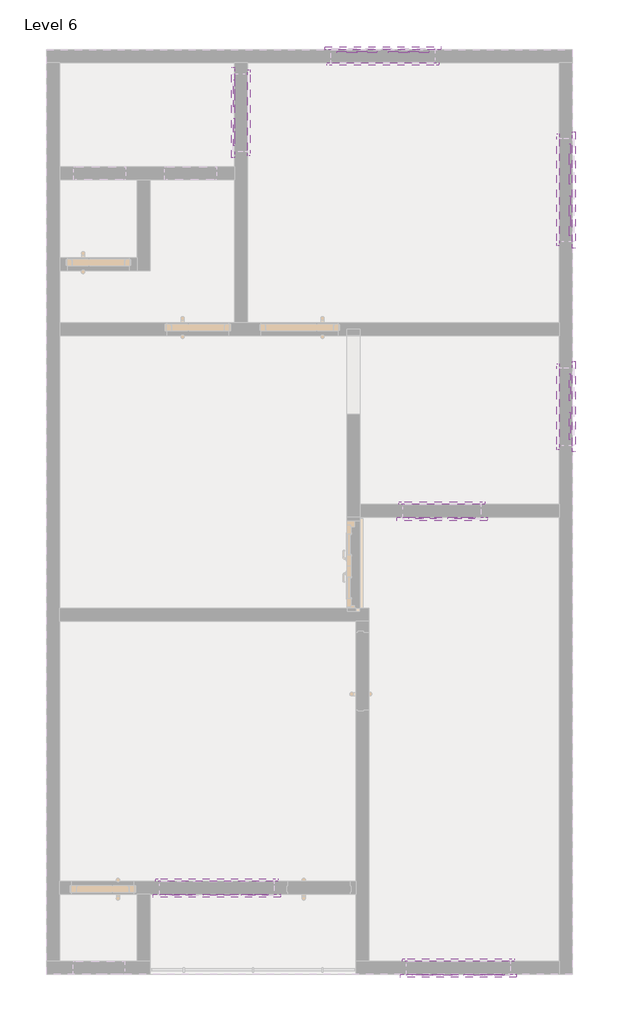
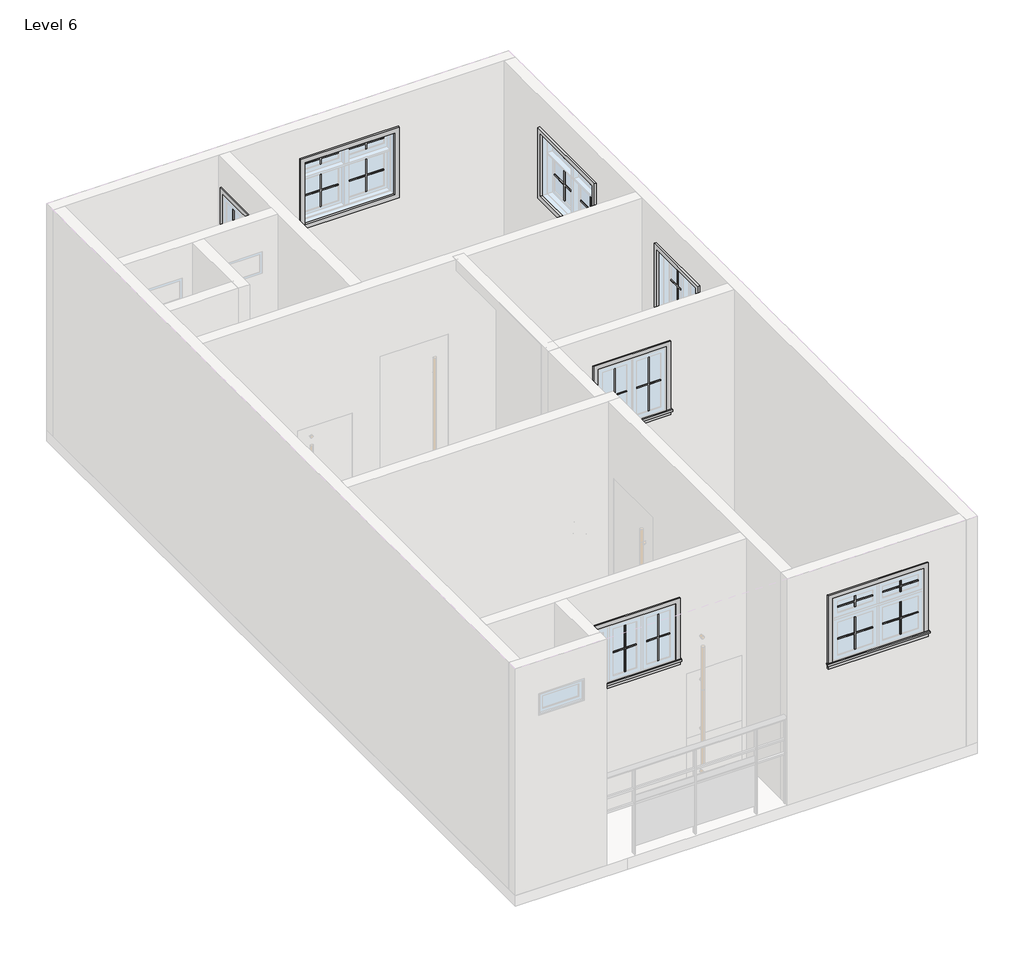
# One storey, part 3 of 3: 74 proxies.
"""IFC4 building model written with IfcOpenShell, lengths in millimetres."""

from ifc_helpers import new_model, si_unit, origin, place, context, project, spatial, transform, mapped, element, save
from components import m_muntin_pattern_2x2_m_muntin_pattern_2x2_ec2ff75e, m_muntin_pattern_2x2_m_muntin_pattern_2x2_6a19bea2, m_muntin_pattern_2x2_m_muntin_pattern_2x2_383df7b3, m_muntin_pattern_2x2_m_muntin_pattern_2x2_55460d9e, m_muntin_pattern_2x2_m_muntin_pattern_2x2_a9b7b7a9, m_muntin_pattern_2x2_m_muntin_pattern_2x2_c959817e, m_muntin_pattern_2x2_m_muntin_pattern_2x2_9259c5e2, m_trim_window_exterior_flat_with_sill_b1b88069, m_trim_window_exterior_flat_with_sill_8fa486dc, m_trim_window_exterior_flat_with_sill_2a9c44ae, m_trim_window_interior_flat_picture_frame_7d12f20c, m_trim_window_interior_flat_picture_frame_b6dd03a6, m_trim_window_interior_flat_picture_frame_c139440e

model = new_model("IFC4")

# Units and contexts
model_context = context("Model", 3, world=origin())
ifc_project = project(units=[si_unit("LENGTHUNIT", "METRE", prefix="MILLI")], contexts=[model_context])

# Site, building, storey
site = spatial("IfcSite", under=ifc_project)
building = spatial("IfcBuilding", under=site)
storey = spatial("IfcBuildingStorey", under=building, Name="Level 6", Elevation=7010.4)

# Proxies
placement = place(None, origin())
m_muntin_pattern_2x2_m_muntin_pattern_2x2_shape = m_muntin_pattern_2x2_m_muntin_pattern_2x2_ec2ff75e(model_context)
element("IfcBuildingElementProxy", 1, Name="M_Muntin Pattern_2x2 : M_Muntin Pattern_2x2", ObjectType="M_Muntin Pattern_2x2 : M_Muntin Pattern_2x2", at=placement, inside=storey, context=model_context, shape_type="MappedRepresentation", body=[
    mapped(m_muntin_pattern_2x2_m_muntin_pattern_2x2_shape, transform((-20164.8088079, 6316.5492053, 8909.05), x_axis=(1.0, 0.0, 0.0), y_axis=(0.0, 1.0, 0.0), z_axis=(0.0, 0.0, 1.0))),
])
element("IfcBuildingElementProxy", 2, Name="M_Muntin Pattern_2x2 : M_Muntin Pattern_2x2", ObjectType="M_Muntin Pattern_2x2 : M_Muntin Pattern_2x2", at=placement, inside=storey, context=model_context, shape_type="MappedRepresentation", body=[
    mapped(m_muntin_pattern_2x2_m_muntin_pattern_2x2_shape, transform((-17648.6213079, 4984.6367053, 8909.05), x_axis=(0.0, -1.0, 0.0), y_axis=(1.0, 0.0, 0.0), z_axis=(0.0, 0.0, 1.0))),
])
element("IfcBuildingElementProxy", 3, Name="M_Muntin Pattern_2x2 : M_Muntin Pattern_2x2", ObjectType="M_Muntin Pattern_2x2 : M_Muntin Pattern_2x2", at=placement, inside=storey, context=model_context, shape_type="MappedRepresentation", body=[
    mapped(m_muntin_pattern_2x2_m_muntin_pattern_2x2_shape, transform((-18672.7572454, -4510.2007947, 8909.05), x_axis=(-1.0, 0.0, 0.0), y_axis=(0.0, -1.0, 0.0), z_axis=(0.0, 0.0, 1.0))),
])
m_muntin_pattern_2x2_m_muntin_pattern_2x2_2_shape = m_muntin_pattern_2x2_m_muntin_pattern_2x2_6a19bea2(model_context)
element("IfcBuildingElementProxy", 4, Name="M_Muntin Pattern_2x2 : M_Muntin Pattern_2x2", ObjectType="M_Muntin Pattern_2x2 : M_Muntin Pattern_2x2", at=placement, inside=storey, context=model_context, shape_type="MappedRepresentation", body=[
    mapped(m_muntin_pattern_2x2_m_muntin_pattern_2x2_2_shape, transform((-19558.3838079, 6316.5492053, 8909.05), x_axis=(-1.0, 0.0, 0.0), y_axis=(0.0, -1.0, 0.0), z_axis=(0.0, 0.0, 1.0))),
])
element("IfcBuildingElementProxy", 5, Name="M_Muntin Pattern_2x2 : M_Muntin Pattern_2x2", ObjectType="M_Muntin Pattern_2x2 : M_Muntin Pattern_2x2", at=placement, inside=storey, context=model_context, shape_type="MappedRepresentation", body=[
    mapped(m_muntin_pattern_2x2_m_muntin_pattern_2x2_2_shape, transform((-17648.6213079, 4378.2117053, 8909.05), x_axis=(0.0, 1.0, 0.0), y_axis=(-1.0, 0.0, 0.0), z_axis=(0.0, 0.0, 1.0))),
])
element("IfcBuildingElementProxy", 6, Name="M_Muntin Pattern_2x2 : M_Muntin Pattern_2x2", ObjectType="M_Muntin Pattern_2x2 : M_Muntin Pattern_2x2", at=placement, inside=storey, context=model_context, shape_type="MappedRepresentation", body=[
    mapped(m_muntin_pattern_2x2_m_muntin_pattern_2x2_2_shape, transform((-19279.1822454, -4510.2007947, 8909.05), x_axis=(1.0, 0.0, 0.0), y_axis=(0.0, 1.0, 0.0), z_axis=(0.0, 0.0, 1.0))),
])
m_muntin_pattern_2x2_m_muntin_pattern_2x2_3_shape = m_muntin_pattern_2x2_m_muntin_pattern_2x2_383df7b3(model_context)
element("IfcBuildingElementProxy", 7, Name="M_Muntin Pattern_2x2 : M_Muntin Pattern_2x2", ObjectType="M_Muntin Pattern_2x2 : M_Muntin Pattern_2x2", at=placement, inside=storey, context=model_context, shape_type="MappedRepresentation", body=[
    mapped(m_muntin_pattern_2x2_m_muntin_pattern_2x2_3_shape, transform((-19558.3838079, 6316.5492053, 9509.05), x_axis=(-1.0, 0.0, 0.0), y_axis=(0.0, -1.0, 0.0), z_axis=(0.0, 0.0, 1.0))),
])
element("IfcBuildingElementProxy", 8, Name="M_Muntin Pattern_2x2 : M_Muntin Pattern_2x2", ObjectType="M_Muntin Pattern_2x2 : M_Muntin Pattern_2x2", at=placement, inside=storey, context=model_context, shape_type="MappedRepresentation", body=[
    mapped(m_muntin_pattern_2x2_m_muntin_pattern_2x2_3_shape, transform((-20164.8088079, 6316.5492053, 9509.05), x_axis=(-1.0, 0.0, 0.0), y_axis=(0.0, -1.0, 0.0), z_axis=(0.0, 0.0, 1.0))),
])
element("IfcBuildingElementProxy", 9, Name="M_Muntin Pattern_2x2 : M_Muntin Pattern_2x2", ObjectType="M_Muntin Pattern_2x2 : M_Muntin Pattern_2x2", at=placement, inside=storey, context=model_context, shape_type="MappedRepresentation", body=[
    mapped(m_muntin_pattern_2x2_m_muntin_pattern_2x2_3_shape, transform((-17648.6213079, 4378.2117053, 9509.05), x_axis=(0.0, 1.0, 0.0), y_axis=(-1.0, 0.0, 0.0), z_axis=(0.0, 0.0, 1.0))),
])
element("IfcBuildingElementProxy", 10, Name="M_Muntin Pattern_2x2 : M_Muntin Pattern_2x2", ObjectType="M_Muntin Pattern_2x2 : M_Muntin Pattern_2x2", at=placement, inside=storey, context=model_context, shape_type="MappedRepresentation", body=[
    mapped(m_muntin_pattern_2x2_m_muntin_pattern_2x2_3_shape, transform((-17648.6213079, 4984.6367053, 9509.05), x_axis=(0.0, 1.0, 0.0), y_axis=(-1.0, 0.0, 0.0), z_axis=(0.0, 0.0, 1.0))),
])
element("IfcBuildingElementProxy", 11, Name="M_Muntin Pattern_2x2 : M_Muntin Pattern_2x2", ObjectType="M_Muntin Pattern_2x2 : M_Muntin Pattern_2x2", at=placement, inside=storey, context=model_context, shape_type="MappedRepresentation", body=[
    mapped(m_muntin_pattern_2x2_m_muntin_pattern_2x2_3_shape, transform((-19279.1822454, -4510.2007947, 9509.05), x_axis=(1.0, 0.0, 0.0), y_axis=(0.0, 1.0, 0.0), z_axis=(0.0, 0.0, 1.0))),
])
element("IfcBuildingElementProxy", 12, Name="M_Muntin Pattern_2x2 : M_Muntin Pattern_2x2", ObjectType="M_Muntin Pattern_2x2 : M_Muntin Pattern_2x2", at=placement, inside=storey, context=model_context, shape_type="MappedRepresentation", body=[
    mapped(m_muntin_pattern_2x2_m_muntin_pattern_2x2_3_shape, transform((-18672.7572454, -4510.2007947, 9509.05), x_axis=(1.0, 0.0, 0.0), y_axis=(0.0, 1.0, 0.0), z_axis=(0.0, 0.0, 1.0))),
])
m_muntin_pattern_2x2_m_muntin_pattern_2x2_4_shape = m_muntin_pattern_2x2_m_muntin_pattern_2x2_55460d9e(model_context)
element("IfcBuildingElementProxy", 13, Name="M_Muntin Pattern_2x2 : M_Muntin Pattern_2x2", ObjectType="M_Muntin Pattern_2x2 : M_Muntin Pattern_2x2", at=placement, inside=storey, context=model_context, shape_type="MappedRepresentation", body=[
    mapped(m_muntin_pattern_2x2_m_muntin_pattern_2x2_4_shape, transform((-18939.9533391, 849.1992053, 8909.05), x_axis=(-1.0, 0.0, 0.0), y_axis=(0.0, -1.0, 0.0), z_axis=(0.0, 0.0, 1.0))),
])
element("IfcBuildingElementProxy", 14, Name="M_Muntin Pattern_2x2 : M_Muntin Pattern_2x2", ObjectType="M_Muntin Pattern_2x2 : M_Muntin Pattern_2x2", at=placement, inside=storey, context=model_context, shape_type="MappedRepresentation", body=[
    mapped(m_muntin_pattern_2x2_m_muntin_pattern_2x2_4_shape, transform((-17648.6213079, 2366.8492053, 8909.05), x_axis=(0.0, -1.0, 0.0), y_axis=(1.0, 0.0, 0.0), z_axis=(0.0, 0.0, 1.0))),
])
element("IfcBuildingElementProxy", 15, Name="M_Muntin Pattern_2x2 : M_Muntin Pattern_2x2", ObjectType="M_Muntin Pattern_2x2 : M_Muntin Pattern_2x2", at=placement, inside=storey, context=model_context, shape_type="MappedRepresentation", body=[
    mapped(m_muntin_pattern_2x2_m_muntin_pattern_2x2_4_shape, transform((-21591.9713079, 5362.4617053, 8909.05), x_axis=(0.0, 1.0, 0.0), y_axis=(-1.0, 0.0, 0.0), z_axis=(0.0, 0.0, 1.0))),
])
element("IfcBuildingElementProxy", 16, Name="M_Muntin Pattern_2x2 : M_Muntin Pattern_2x2", ObjectType="M_Muntin Pattern_2x2 : M_Muntin Pattern_2x2", at=placement, inside=storey, context=model_context, shape_type="MappedRepresentation", body=[
    mapped(m_muntin_pattern_2x2_m_muntin_pattern_2x2_4_shape, transform((-18939.9533391, 849.1992053, 8909.05), x_axis=(-1.0, 0.0, 0.0), y_axis=(0.0, -1.0, 0.0), z_axis=(0.0, 0.0, 1.0))),
])
element("IfcBuildingElementProxy", 17, Name="M_Muntin Pattern_2x2 : M_Muntin Pattern_2x2", ObjectType="M_Muntin Pattern_2x2 : M_Muntin Pattern_2x2", at=placement, inside=storey, context=model_context, shape_type="MappedRepresentation", body=[
    mapped(m_muntin_pattern_2x2_m_muntin_pattern_2x2_4_shape, transform((-21591.9713079, 5362.4617053, 8909.05), x_axis=(0.0, 1.0, 0.0), y_axis=(-1.0, 0.0, 0.0), z_axis=(0.0, 0.0, 1.0))),
])
element("IfcBuildingElementProxy", 18, Name="M_Muntin Pattern_2x2 : M_Muntin Pattern_2x2", ObjectType="M_Muntin Pattern_2x2 : M_Muntin Pattern_2x2", at=placement, inside=storey, context=model_context, shape_type="MappedRepresentation", body=[
    mapped(m_muntin_pattern_2x2_m_muntin_pattern_2x2_4_shape, transform((-18939.9533391, 849.1992053, 8909.05), x_axis=(-1.0, 0.0, 0.0), y_axis=(0.0, -1.0, 0.0), z_axis=(0.0, 0.0, 1.0))),
])
element("IfcBuildingElementProxy", 19, Name="M_Muntin Pattern_2x2 : M_Muntin Pattern_2x2", ObjectType="M_Muntin Pattern_2x2 : M_Muntin Pattern_2x2", at=placement, inside=storey, context=model_context, shape_type="MappedRepresentation", body=[
    mapped(m_muntin_pattern_2x2_m_muntin_pattern_2x2_4_shape, transform((-21591.9713079, 5362.4617053, 8909.05), x_axis=(0.0, 1.0, 0.0), y_axis=(-1.0, 0.0, 0.0), z_axis=(0.0, 0.0, 1.0))),
])
element("IfcBuildingElementProxy", 20, Name="M_Muntin Pattern_2x2 : M_Muntin Pattern_2x2", ObjectType="M_Muntin Pattern_2x2 : M_Muntin Pattern_2x2", at=placement, inside=storey, context=model_context, shape_type="MappedRepresentation", body=[
    mapped(m_muntin_pattern_2x2_m_muntin_pattern_2x2_4_shape, transform((-18939.9533391, 849.1992053, 8909.05), x_axis=(-1.0, 0.0, 0.0), y_axis=(0.0, -1.0, 0.0), z_axis=(0.0, 0.0, 1.0))),
])
element("IfcBuildingElementProxy", 21, Name="M_Muntin Pattern_2x2 : M_Muntin Pattern_2x2", ObjectType="M_Muntin Pattern_2x2 : M_Muntin Pattern_2x2", at=placement, inside=storey, context=model_context, shape_type="MappedRepresentation", body=[
    mapped(m_muntin_pattern_2x2_m_muntin_pattern_2x2_4_shape, transform((-21591.9713079, 5362.4617053, 8909.05), x_axis=(0.0, 1.0, 0.0), y_axis=(-1.0, 0.0, 0.0), z_axis=(0.0, 0.0, 1.0))),
])
m_muntin_pattern_2x2_m_muntin_pattern_2x2_5_shape = m_muntin_pattern_2x2_m_muntin_pattern_2x2_a9b7b7a9(model_context)
element("IfcBuildingElementProxy", 22, Name="M_Muntin Pattern_2x2 : M_Muntin Pattern_2x2", ObjectType="M_Muntin Pattern_2x2 : M_Muntin Pattern_2x2", at=placement, inside=storey, context=model_context, shape_type="MappedRepresentation", body=[
    mapped(m_muntin_pattern_2x2_m_muntin_pattern_2x2_5_shape, transform((-19393.9783391, 849.1992053, 8909.05), x_axis=(1.0, 0.0, 0.0), y_axis=(0.0, 1.0, 0.0), z_axis=(0.0, 0.0, 1.0))),
])
element("IfcBuildingElementProxy", 23, Name="M_Muntin Pattern_2x2 : M_Muntin Pattern_2x2", ObjectType="M_Muntin Pattern_2x2 : M_Muntin Pattern_2x2", at=placement, inside=storey, context=model_context, shape_type="MappedRepresentation", body=[
    mapped(m_muntin_pattern_2x2_m_muntin_pattern_2x2_5_shape, transform((-17648.6213079, 1912.8242053, 8909.05), x_axis=(0.0, 1.0, 0.0), y_axis=(-1.0, 0.0, 0.0), z_axis=(0.0, 0.0, 1.0))),
])
element("IfcBuildingElementProxy", 24, Name="M_Muntin Pattern_2x2 : M_Muntin Pattern_2x2", ObjectType="M_Muntin Pattern_2x2 : M_Muntin Pattern_2x2", at=placement, inside=storey, context=model_context, shape_type="MappedRepresentation", body=[
    mapped(m_muntin_pattern_2x2_m_muntin_pattern_2x2_5_shape, transform((-21591.9713079, 5816.4867053, 8909.05), x_axis=(0.0, -1.0, 0.0), y_axis=(1.0, 0.0, 0.0), z_axis=(0.0, 0.0, 1.0))),
])
element("IfcBuildingElementProxy", 25, Name="M_Muntin Pattern_2x2 : M_Muntin Pattern_2x2", ObjectType="M_Muntin Pattern_2x2 : M_Muntin Pattern_2x2", at=placement, inside=storey, context=model_context, shape_type="MappedRepresentation", body=[
    mapped(m_muntin_pattern_2x2_m_muntin_pattern_2x2_5_shape, transform((-19393.9783391, 849.1992053, 8909.05), x_axis=(1.0, 0.0, 0.0), y_axis=(0.0, 1.0, 0.0), z_axis=(0.0, 0.0, 1.0))),
])
element("IfcBuildingElementProxy", 26, Name="M_Muntin Pattern_2x2 : M_Muntin Pattern_2x2", ObjectType="M_Muntin Pattern_2x2 : M_Muntin Pattern_2x2", at=placement, inside=storey, context=model_context, shape_type="MappedRepresentation", body=[
    mapped(m_muntin_pattern_2x2_m_muntin_pattern_2x2_5_shape, transform((-21591.9713079, 5816.4867053, 8909.05), x_axis=(0.0, -1.0, 0.0), y_axis=(1.0, 0.0, 0.0), z_axis=(0.0, 0.0, 1.0))),
])
element("IfcBuildingElementProxy", 27, Name="M_Muntin Pattern_2x2 : M_Muntin Pattern_2x2", ObjectType="M_Muntin Pattern_2x2 : M_Muntin Pattern_2x2", at=placement, inside=storey, context=model_context, shape_type="MappedRepresentation", body=[
    mapped(m_muntin_pattern_2x2_m_muntin_pattern_2x2_5_shape, transform((-19393.9783391, 849.1992053, 8909.05), x_axis=(1.0, 0.0, 0.0), y_axis=(0.0, 1.0, 0.0), z_axis=(0.0, 0.0, 1.0))),
])
element("IfcBuildingElementProxy", 28, Name="M_Muntin Pattern_2x2 : M_Muntin Pattern_2x2", ObjectType="M_Muntin Pattern_2x2 : M_Muntin Pattern_2x2", at=placement, inside=storey, context=model_context, shape_type="MappedRepresentation", body=[
    mapped(m_muntin_pattern_2x2_m_muntin_pattern_2x2_5_shape, transform((-21591.9713079, 5816.4867053, 8909.05), x_axis=(0.0, -1.0, 0.0), y_axis=(1.0, 0.0, 0.0), z_axis=(0.0, 0.0, 1.0))),
])
element("IfcBuildingElementProxy", 29, Name="M_Muntin Pattern_2x2 : M_Muntin Pattern_2x2", ObjectType="M_Muntin Pattern_2x2 : M_Muntin Pattern_2x2", at=placement, inside=storey, context=model_context, shape_type="MappedRepresentation", body=[
    mapped(m_muntin_pattern_2x2_m_muntin_pattern_2x2_5_shape, transform((-19393.9783391, 849.1992053, 8909.05), x_axis=(1.0, 0.0, 0.0), y_axis=(0.0, 1.0, 0.0), z_axis=(0.0, 0.0, 1.0))),
])
element("IfcBuildingElementProxy", 30, Name="M_Muntin Pattern_2x2 : M_Muntin Pattern_2x2", ObjectType="M_Muntin Pattern_2x2 : M_Muntin Pattern_2x2", at=placement, inside=storey, context=model_context, shape_type="MappedRepresentation", body=[
    mapped(m_muntin_pattern_2x2_m_muntin_pattern_2x2_5_shape, transform((-21591.9713079, 5816.4867053, 8909.05), x_axis=(0.0, -1.0, 0.0), y_axis=(1.0, 0.0, 0.0), z_axis=(0.0, 0.0, 1.0))),
])
m_muntin_pattern_2x2_m_muntin_pattern_2x2_6_shape = m_muntin_pattern_2x2_m_muntin_pattern_2x2_c959817e(model_context)
element("IfcBuildingElementProxy", 31, Name="M_Muntin Pattern_2x2 : M_Muntin Pattern_2x2", ObjectType="M_Muntin Pattern_2x2 : M_Muntin Pattern_2x2", at=placement, inside=storey, context=model_context, shape_type="MappedRepresentation", body=[
    mapped(m_muntin_pattern_2x2_m_muntin_pattern_2x2_6_shape, transform((-21364.4296412, -3570.4007947, 8909.05), x_axis=(-1.0, 0.0, 0.0), y_axis=(0.0, -1.0, 0.0), z_axis=(0.0, 0.0, 1.0))),
])
element("IfcBuildingElementProxy", 32, Name="M_Muntin Pattern_2x2 : M_Muntin Pattern_2x2", ObjectType="M_Muntin Pattern_2x2 : M_Muntin Pattern_2x2", at=placement, inside=storey, context=model_context, shape_type="MappedRepresentation", body=[
    mapped(m_muntin_pattern_2x2_m_muntin_pattern_2x2_6_shape, transform((-21364.4296412, -3570.4007947, 8909.05), x_axis=(-1.0, 0.0, 0.0), y_axis=(0.0, -1.0, 0.0), z_axis=(0.0, 0.0, 1.0))),
])
element("IfcBuildingElementProxy", 33, Name="M_Muntin Pattern_2x2 : M_Muntin Pattern_2x2", ObjectType="M_Muntin Pattern_2x2 : M_Muntin Pattern_2x2", at=placement, inside=storey, context=model_context, shape_type="MappedRepresentation", body=[
    mapped(m_muntin_pattern_2x2_m_muntin_pattern_2x2_6_shape, transform((-21364.4296412, -3570.4007947, 8909.05), x_axis=(-1.0, 0.0, 0.0), y_axis=(0.0, -1.0, 0.0), z_axis=(0.0, 0.0, 1.0))),
])
element("IfcBuildingElementProxy", 34, Name="M_Muntin Pattern_2x2 : M_Muntin Pattern_2x2", ObjectType="M_Muntin Pattern_2x2 : M_Muntin Pattern_2x2", at=placement, inside=storey, context=model_context, shape_type="MappedRepresentation", body=[
    mapped(m_muntin_pattern_2x2_m_muntin_pattern_2x2_6_shape, transform((-21364.4296412, -3570.4007947, 8909.05), x_axis=(-1.0, 0.0, 0.0), y_axis=(0.0, -1.0, 0.0), z_axis=(0.0, 0.0, 1.0))),
])
m_muntin_pattern_2x2_m_muntin_pattern_2x2_7_shape = m_muntin_pattern_2x2_m_muntin_pattern_2x2_9259c5e2(model_context)
element("IfcBuildingElementProxy", 35, Name="M_Muntin Pattern_2x2 : M_Muntin Pattern_2x2", ObjectType="M_Muntin Pattern_2x2 : M_Muntin Pattern_2x2", at=placement, inside=storey, context=model_context, shape_type="MappedRepresentation", body=[
    mapped(m_muntin_pattern_2x2_m_muntin_pattern_2x2_7_shape, transform((-22257.6629746, -3570.4007947, 8909.05), x_axis=(1.0, 0.0, 0.0), y_axis=(0.0, 1.0, 0.0), z_axis=(0.0, 0.0, 1.0))),
])
element("IfcBuildingElementProxy", 36, Name="M_Muntin Pattern_2x2 : M_Muntin Pattern_2x2", ObjectType="M_Muntin Pattern_2x2 : M_Muntin Pattern_2x2", at=placement, inside=storey, context=model_context, shape_type="MappedRepresentation", body=[
    mapped(m_muntin_pattern_2x2_m_muntin_pattern_2x2_7_shape, transform((-21811.0463079, -3570.4007947, 8909.05), x_axis=(1.0, 0.0, 0.0), y_axis=(0.0, 1.0, 0.0), z_axis=(0.0, 0.0, 1.0))),
])
element("IfcBuildingElementProxy", 37, Name="M_Muntin Pattern_2x2 : M_Muntin Pattern_2x2", ObjectType="M_Muntin Pattern_2x2 : M_Muntin Pattern_2x2", at=placement, inside=storey, context=model_context, shape_type="MappedRepresentation", body=[
    mapped(m_muntin_pattern_2x2_m_muntin_pattern_2x2_7_shape, transform((-22257.6629746, -3570.4007947, 8909.05), x_axis=(1.0, 0.0, 0.0), y_axis=(0.0, 1.0, 0.0), z_axis=(0.0, 0.0, 1.0))),
])
element("IfcBuildingElementProxy", 38, Name="M_Muntin Pattern_2x2 : M_Muntin Pattern_2x2", ObjectType="M_Muntin Pattern_2x2 : M_Muntin Pattern_2x2", at=placement, inside=storey, context=model_context, shape_type="MappedRepresentation", body=[
    mapped(m_muntin_pattern_2x2_m_muntin_pattern_2x2_7_shape, transform((-21811.0463079, -3570.4007947, 8909.05), x_axis=(1.0, 0.0, 0.0), y_axis=(0.0, 1.0, 0.0), z_axis=(0.0, 0.0, 1.0))),
])
element("IfcBuildingElementProxy", 39, Name="M_Muntin Pattern_2x2 : M_Muntin Pattern_2x2", ObjectType="M_Muntin Pattern_2x2 : M_Muntin Pattern_2x2", at=placement, inside=storey, context=model_context, shape_type="MappedRepresentation", body=[
    mapped(m_muntin_pattern_2x2_m_muntin_pattern_2x2_7_shape, transform((-22257.6629746, -3570.4007947, 8909.05), x_axis=(1.0, 0.0, 0.0), y_axis=(0.0, 1.0, 0.0), z_axis=(0.0, 0.0, 1.0))),
])
element("IfcBuildingElementProxy", 40, Name="M_Muntin Pattern_2x2 : M_Muntin Pattern_2x2", ObjectType="M_Muntin Pattern_2x2 : M_Muntin Pattern_2x2", at=placement, inside=storey, context=model_context, shape_type="MappedRepresentation", body=[
    mapped(m_muntin_pattern_2x2_m_muntin_pattern_2x2_7_shape, transform((-21811.0463079, -3570.4007947, 8909.05), x_axis=(1.0, 0.0, 0.0), y_axis=(0.0, 1.0, 0.0), z_axis=(0.0, 0.0, 1.0))),
])
element("IfcBuildingElementProxy", 41, Name="M_Muntin Pattern_2x2 : M_Muntin Pattern_2x2", ObjectType="M_Muntin Pattern_2x2 : M_Muntin Pattern_2x2", at=placement, inside=storey, context=model_context, shape_type="MappedRepresentation", body=[
    mapped(m_muntin_pattern_2x2_m_muntin_pattern_2x2_7_shape, transform((-22257.6629746, -3570.4007947, 8909.05), x_axis=(1.0, 0.0, 0.0), y_axis=(0.0, 1.0, 0.0), z_axis=(0.0, 0.0, 1.0))),
])
element("IfcBuildingElementProxy", 42, Name="M_Muntin Pattern_2x2 : M_Muntin Pattern_2x2", ObjectType="M_Muntin Pattern_2x2 : M_Muntin Pattern_2x2", at=placement, inside=storey, context=model_context, shape_type="MappedRepresentation", body=[
    mapped(m_muntin_pattern_2x2_m_muntin_pattern_2x2_7_shape, transform((-21811.0463079, -3570.4007947, 8909.05), x_axis=(1.0, 0.0, 0.0), y_axis=(0.0, 1.0, 0.0), z_axis=(0.0, 0.0, 1.0))),
])
m_trim_window_exterior_flat_with_sill_shape = m_trim_window_exterior_flat_with_sill_b1b88069(model_context)
element("IfcBuildingElementProxy", 43, Name="M_Trim-Window-Exterior-Flat : with Sill", ObjectType="M_Trim-Window-Exterior-Flat : with Sill", at=placement, inside=storey, context=model_context, shape_type="MappedRepresentation", body=[
    mapped(m_trim_window_exterior_flat_with_sill_shape, transform((-19861.5963079, 6326.0742053, 9739.2), x_axis=(-1.0, 0.0, 0.0), y_axis=(0.0, 0.0, 1.0), z_axis=(0.0, 1.0, 0.0))),
])
element("IfcBuildingElementProxy", 44, Name="M_Trim-Window-Exterior-Flat : with Sill", ObjectType="M_Trim-Window-Exterior-Flat : with Sill", at=placement, inside=storey, context=model_context, shape_type="MappedRepresentation", body=[
    mapped(m_trim_window_exterior_flat_with_sill_shape, transform((-17639.0963079, 4681.4242053, 9739.2), x_axis=(0.0, 1.0, 0.0), y_axis=(0.0, 0.0, 1.0), z_axis=(1.0, 0.0, 0.0))),
])
element("IfcBuildingElementProxy", 45, Name="M_Trim-Window-Exterior-Flat : with Sill", ObjectType="M_Trim-Window-Exterior-Flat : with Sill", at=placement, inside=storey, context=model_context, shape_type="MappedRepresentation", body=[
    mapped(m_trim_window_exterior_flat_with_sill_shape, transform((-18975.9697454, -4519.7257947, 9739.2), x_axis=(1.0, 0.0, 0.0), y_axis=(0.0, 0.0, 1.0), z_axis=(0.0, -1.0, 0.0))),
])
m_trim_window_exterior_flat_with_sill_2_shape = m_trim_window_exterior_flat_with_sill_8fa486dc(model_context)
element("IfcBuildingElementProxy", 46, Name="M_Trim-Window-Exterior-Flat : with Sill", ObjectType="M_Trim-Window-Exterior-Flat : with Sill", at=placement, inside=storey, context=model_context, shape_type="MappedRepresentation", body=[
    mapped(m_trim_window_exterior_flat_with_sill_2_shape, transform((-19166.9658391, 839.6742053, 9739.2), x_axis=(1.0, 0.0, 0.0), y_axis=(0.0, 0.0, 1.0), z_axis=(0.0, -1.0, 0.0))),
])
element("IfcBuildingElementProxy", 47, Name="M_Trim-Window-Exterior-Flat : with Sill", ObjectType="M_Trim-Window-Exterior-Flat : with Sill", at=placement, inside=storey, context=model_context, shape_type="MappedRepresentation", body=[
    mapped(m_trim_window_exterior_flat_with_sill_2_shape, transform((-17639.0963079, 2139.8367053, 9739.2), x_axis=(0.0, 1.0, 0.0), y_axis=(0.0, 0.0, 1.0), z_axis=(1.0, 0.0, 0.0))),
])
element("IfcBuildingElementProxy", 48, Name="M_Trim-Window-Exterior-Flat : with Sill", ObjectType="M_Trim-Window-Exterior-Flat : with Sill", at=placement, inside=storey, context=model_context, shape_type="MappedRepresentation", body=[
    mapped(m_trim_window_exterior_flat_with_sill_2_shape, transform((-21601.4963079, 5589.4742053, 9739.2), x_axis=(0.0, -1.0, 0.0), y_axis=(0.0, 0.0, 1.0), z_axis=(-1.0, 0.0, 0.0))),
])
element("IfcBuildingElementProxy", 49, Name="M_Trim-Window-Exterior-Flat : with Sill", ObjectType="M_Trim-Window-Exterior-Flat : with Sill", at=placement, inside=storey, context=model_context, shape_type="MappedRepresentation", body=[
    mapped(m_trim_window_exterior_flat_with_sill_2_shape, transform((-19166.9658391, 839.6742053, 9739.2), x_axis=(1.0, 0.0, 0.0), y_axis=(0.0, 0.0, 1.0), z_axis=(0.0, -1.0, 0.0))),
])
element("IfcBuildingElementProxy", 50, Name="M_Trim-Window-Exterior-Flat : with Sill", ObjectType="M_Trim-Window-Exterior-Flat : with Sill", at=placement, inside=storey, context=model_context, shape_type="MappedRepresentation", body=[
    mapped(m_trim_window_exterior_flat_with_sill_2_shape, transform((-21601.4963079, 5589.4742053, 9739.2), x_axis=(0.0, -1.0, 0.0), y_axis=(0.0, 0.0, 1.0), z_axis=(-1.0, 0.0, 0.0))),
])
element("IfcBuildingElementProxy", 51, Name="M_Trim-Window-Exterior-Flat : with Sill", ObjectType="M_Trim-Window-Exterior-Flat : with Sill", at=placement, inside=storey, context=model_context, shape_type="MappedRepresentation", body=[
    mapped(m_trim_window_exterior_flat_with_sill_2_shape, transform((-19166.9658391, 839.6742053, 9739.2), x_axis=(1.0, 0.0, 0.0), y_axis=(0.0, 0.0, 1.0), z_axis=(0.0, -1.0, 0.0))),
])
element("IfcBuildingElementProxy", 52, Name="M_Trim-Window-Exterior-Flat : with Sill", ObjectType="M_Trim-Window-Exterior-Flat : with Sill", at=placement, inside=storey, context=model_context, shape_type="MappedRepresentation", body=[
    mapped(m_trim_window_exterior_flat_with_sill_2_shape, transform((-21601.4963079, 5589.4742053, 9739.2), x_axis=(0.0, -1.0, 0.0), y_axis=(0.0, 0.0, 1.0), z_axis=(-1.0, 0.0, 0.0))),
])
element("IfcBuildingElementProxy", 53, Name="M_Trim-Window-Exterior-Flat : with Sill", ObjectType="M_Trim-Window-Exterior-Flat : with Sill", at=placement, inside=storey, context=model_context, shape_type="MappedRepresentation", body=[
    mapped(m_trim_window_exterior_flat_with_sill_2_shape, transform((-19166.9658391, 839.6742053, 9739.2), x_axis=(1.0, 0.0, 0.0), y_axis=(0.0, 0.0, 1.0), z_axis=(0.0, -1.0, 0.0))),
])
element("IfcBuildingElementProxy", 54, Name="M_Trim-Window-Exterior-Flat : with Sill", ObjectType="M_Trim-Window-Exterior-Flat : with Sill", at=placement, inside=storey, context=model_context, shape_type="MappedRepresentation", body=[
    mapped(m_trim_window_exterior_flat_with_sill_2_shape, transform((-21601.4963079, 5589.4742053, 9739.2), x_axis=(0.0, -1.0, 0.0), y_axis=(0.0, 0.0, 1.0), z_axis=(-1.0, 0.0, 0.0))),
])
m_trim_window_exterior_flat_with_sill_3_shape = m_trim_window_exterior_flat_with_sill_2a9c44ae(model_context)
element("IfcBuildingElementProxy", 55, Name="M_Trim-Window-Exterior-Flat : with Sill", ObjectType="M_Trim-Window-Exterior-Flat : with Sill", at=placement, inside=storey, context=model_context, shape_type="MappedRepresentation", body=[
    mapped(m_trim_window_exterior_flat_with_sill_3_shape, transform((-21811.0463079, -3579.9257947, 9639.2), x_axis=(1.0, 0.0, 0.0), y_axis=(0.0, 0.0, 1.0), z_axis=(0.0, -1.0, 0.0))),
])
element("IfcBuildingElementProxy", 56, Name="M_Trim-Window-Exterior-Flat : with Sill", ObjectType="M_Trim-Window-Exterior-Flat : with Sill", at=placement, inside=storey, context=model_context, shape_type="MappedRepresentation", body=[
    mapped(m_trim_window_exterior_flat_with_sill_3_shape, transform((-21811.0463079, -3579.9257947, 9639.2), x_axis=(1.0, 0.0, 0.0), y_axis=(0.0, 0.0, 1.0), z_axis=(0.0, -1.0, 0.0))),
])
element("IfcBuildingElementProxy", 57, Name="M_Trim-Window-Exterior-Flat : with Sill", ObjectType="M_Trim-Window-Exterior-Flat : with Sill", at=placement, inside=storey, context=model_context, shape_type="MappedRepresentation", body=[
    mapped(m_trim_window_exterior_flat_with_sill_3_shape, transform((-21811.0463079, -3579.9257947, 9639.2), x_axis=(1.0, 0.0, 0.0), y_axis=(0.0, 0.0, 1.0), z_axis=(0.0, -1.0, 0.0))),
])
element("IfcBuildingElementProxy", 58, Name="M_Trim-Window-Exterior-Flat : with Sill", ObjectType="M_Trim-Window-Exterior-Flat : with Sill", at=placement, inside=storey, context=model_context, shape_type="MappedRepresentation", body=[
    mapped(m_trim_window_exterior_flat_with_sill_3_shape, transform((-21811.0463079, -3579.9257947, 9639.2), x_axis=(1.0, 0.0, 0.0), y_axis=(0.0, 0.0, 1.0), z_axis=(0.0, -1.0, 0.0))),
])
m_trim_window_interior_flat_picture_frame_shape = m_trim_window_interior_flat_picture_frame_7d12f20c(model_context)
element("IfcBuildingElementProxy", 59, Name="M_Trim-Window-Interior-Flat : Picture Frame", ObjectType="M_Trim-Window-Interior-Flat : Picture Frame", at=placement, inside=storey, context=model_context, shape_type="MappedRepresentation", body=[
    mapped(m_trim_window_interior_flat_picture_frame_shape, transform((-19861.5963079, 6173.6742053, 9739.2), x_axis=(1.0, 0.0, 0.0), y_axis=(0.0, 0.0, 1.0), z_axis=(0.0, -1.0, 0.0))),
])
element("IfcBuildingElementProxy", 60, Name="M_Trim-Window-Interior-Flat : Picture Frame", ObjectType="M_Trim-Window-Interior-Flat : Picture Frame", at=placement, inside=storey, context=model_context, shape_type="MappedRepresentation", body=[
    mapped(m_trim_window_interior_flat_picture_frame_shape, transform((-17791.4963079, 4681.4242053, 9739.2), x_axis=(0.0, -1.0, 0.0), y_axis=(0.0, 0.0, 1.0), z_axis=(-1.0, 0.0, 0.0))),
])
element("IfcBuildingElementProxy", 61, Name="M_Trim-Window-Interior-Flat : Picture Frame", ObjectType="M_Trim-Window-Interior-Flat : Picture Frame", at=placement, inside=storey, context=model_context, shape_type="MappedRepresentation", body=[
    mapped(m_trim_window_interior_flat_picture_frame_shape, transform((-18975.9697454, -4367.3257947, 9739.2), x_axis=(-1.0, 0.0, 0.0), y_axis=(0.0, 0.0, 1.0), z_axis=(0.0, 1.0, 0.0))),
])
m_trim_window_interior_flat_picture_frame_2_shape = m_trim_window_interior_flat_picture_frame_b6dd03a6(model_context)
element("IfcBuildingElementProxy", 62, Name="M_Trim-Window-Interior-Flat : Picture Frame", ObjectType="M_Trim-Window-Interior-Flat : Picture Frame", at=placement, inside=storey, context=model_context, shape_type="MappedRepresentation", body=[
    mapped(m_trim_window_interior_flat_picture_frame_2_shape, transform((-19166.9658391, 992.0742053, 9739.2), x_axis=(-1.0, 0.0, 0.0), y_axis=(0.0, 0.0, 1.0), z_axis=(0.0, 1.0, 0.0))),
])
element("IfcBuildingElementProxy", 63, Name="M_Trim-Window-Interior-Flat : Picture Frame", ObjectType="M_Trim-Window-Interior-Flat : Picture Frame", at=placement, inside=storey, context=model_context, shape_type="MappedRepresentation", body=[
    mapped(m_trim_window_interior_flat_picture_frame_2_shape, transform((-17791.4963079, 2139.8367053, 9739.2), x_axis=(0.0, -1.0, 0.0), y_axis=(0.0, 0.0, 1.0), z_axis=(-1.0, 0.0, 0.0))),
])
element("IfcBuildingElementProxy", 64, Name="M_Trim-Window-Interior-Flat : Picture Frame", ObjectType="M_Trim-Window-Interior-Flat : Picture Frame", at=placement, inside=storey, context=model_context, shape_type="MappedRepresentation", body=[
    mapped(m_trim_window_interior_flat_picture_frame_2_shape, transform((-21449.0963079, 5589.4742053, 9739.2), x_axis=(0.0, 1.0, 0.0), y_axis=(0.0, 0.0, 1.0), z_axis=(1.0, 0.0, 0.0))),
])
element("IfcBuildingElementProxy", 65, Name="M_Trim-Window-Interior-Flat : Picture Frame", ObjectType="M_Trim-Window-Interior-Flat : Picture Frame", at=placement, inside=storey, context=model_context, shape_type="MappedRepresentation", body=[
    mapped(m_trim_window_interior_flat_picture_frame_2_shape, transform((-19166.9658391, 992.0742053, 9739.2), x_axis=(-1.0, 0.0, 0.0), y_axis=(0.0, 0.0, 1.0), z_axis=(0.0, 1.0, 0.0))),
])
element("IfcBuildingElementProxy", 66, Name="M_Trim-Window-Interior-Flat : Picture Frame", ObjectType="M_Trim-Window-Interior-Flat : Picture Frame", at=placement, inside=storey, context=model_context, shape_type="MappedRepresentation", body=[
    mapped(m_trim_window_interior_flat_picture_frame_2_shape, transform((-21449.0963079, 5589.4742053, 9739.2), x_axis=(0.0, 1.0, 0.0), y_axis=(0.0, 0.0, 1.0), z_axis=(1.0, 0.0, 0.0))),
])
element("IfcBuildingElementProxy", 67, Name="M_Trim-Window-Interior-Flat : Picture Frame", ObjectType="M_Trim-Window-Interior-Flat : Picture Frame", at=placement, inside=storey, context=model_context, shape_type="MappedRepresentation", body=[
    mapped(m_trim_window_interior_flat_picture_frame_2_shape, transform((-19166.9658391, 992.0742053, 9739.2), x_axis=(-1.0, 0.0, 0.0), y_axis=(0.0, 0.0, 1.0), z_axis=(0.0, 1.0, 0.0))),
])
element("IfcBuildingElementProxy", 68, Name="M_Trim-Window-Interior-Flat : Picture Frame", ObjectType="M_Trim-Window-Interior-Flat : Picture Frame", at=placement, inside=storey, context=model_context, shape_type="MappedRepresentation", body=[
    mapped(m_trim_window_interior_flat_picture_frame_2_shape, transform((-21449.0963079, 5589.4742053, 9739.2), x_axis=(0.0, 1.0, 0.0), y_axis=(0.0, 0.0, 1.0), z_axis=(1.0, 0.0, 0.0))),
])
element("IfcBuildingElementProxy", 69, Name="M_Trim-Window-Interior-Flat : Picture Frame", ObjectType="M_Trim-Window-Interior-Flat : Picture Frame", at=placement, inside=storey, context=model_context, shape_type="MappedRepresentation", body=[
    mapped(m_trim_window_interior_flat_picture_frame_2_shape, transform((-19166.9658391, 992.0742053, 9739.2), x_axis=(-1.0, 0.0, 0.0), y_axis=(0.0, 0.0, 1.0), z_axis=(0.0, 1.0, 0.0))),
])
element("IfcBuildingElementProxy", 70, Name="M_Trim-Window-Interior-Flat : Picture Frame", ObjectType="M_Trim-Window-Interior-Flat : Picture Frame", at=placement, inside=storey, context=model_context, shape_type="MappedRepresentation", body=[
    mapped(m_trim_window_interior_flat_picture_frame_2_shape, transform((-21449.0963079, 5589.4742053, 9739.2), x_axis=(0.0, 1.0, 0.0), y_axis=(0.0, 0.0, 1.0), z_axis=(1.0, 0.0, 0.0))),
])
m_trim_window_interior_flat_picture_frame_3_shape = m_trim_window_interior_flat_picture_frame_c139440e(model_context)
element("IfcBuildingElementProxy", 71, Name="M_Trim-Window-Interior-Flat : Picture Frame", ObjectType="M_Trim-Window-Interior-Flat : Picture Frame", at=placement, inside=storey, context=model_context, shape_type="MappedRepresentation", body=[
    mapped(m_trim_window_interior_flat_picture_frame_3_shape, transform((-21811.0463079, -3427.5257947, 9639.2), x_axis=(-1.0, 0.0, 0.0), y_axis=(0.0, 0.0, 1.0), z_axis=(0.0, 1.0, 0.0))),
])
element("IfcBuildingElementProxy", 72, Name="M_Trim-Window-Interior-Flat : Picture Frame", ObjectType="M_Trim-Window-Interior-Flat : Picture Frame", at=placement, inside=storey, context=model_context, shape_type="MappedRepresentation", body=[
    mapped(m_trim_window_interior_flat_picture_frame_3_shape, transform((-21811.0463079, -3427.5257947, 9639.2), x_axis=(-1.0, 0.0, 0.0), y_axis=(0.0, 0.0, 1.0), z_axis=(0.0, 1.0, 0.0))),
])
element("IfcBuildingElementProxy", 73, Name="M_Trim-Window-Interior-Flat : Picture Frame", ObjectType="M_Trim-Window-Interior-Flat : Picture Frame", at=placement, inside=storey, context=model_context, shape_type="MappedRepresentation", body=[
    mapped(m_trim_window_interior_flat_picture_frame_3_shape, transform((-21811.0463079, -3427.5257947, 9639.2), x_axis=(-1.0, 0.0, 0.0), y_axis=(0.0, 0.0, 1.0), z_axis=(0.0, 1.0, 0.0))),
])
element("IfcBuildingElementProxy", 74, Name="M_Trim-Window-Interior-Flat : Picture Frame", ObjectType="M_Trim-Window-Interior-Flat : Picture Frame", at=placement, inside=storey, context=model_context, shape_type="MappedRepresentation", body=[
    mapped(m_trim_window_interior_flat_picture_frame_3_shape, transform((-21811.0463079, -3427.5257947, 9639.2), x_axis=(-1.0, 0.0, 0.0), y_axis=(0.0, 0.0, 1.0), z_axis=(0.0, 1.0, 0.0))),
])

save(model, "model.ifc")

# Revit data of these elements
# Type "M_Muntin Pattern_2x2 : M_Muntin Pattern_2x2"
#   Width [instance default] = 3' - 11.24409"
#   Thickness = 0' - 0 1/2"
#   Height [instance default] = 3' - 11.24409"
#   Distance = 0' - 0 3/4"
#   Interior Material [instance default] = none
#   Exterior Material [instance default] = none
#   Default Elevation = 0
# Type "M_Trim-Window-Exterior-Flat : with Sill"
#   Trim Width = 0' - 2.3622"
#   Trim Thickness_Picture Frame = 0' - 1.1811"
#   Trim Thickness_with Sill = 0' - 0 3/4"
#   Sill Thickness = 0' - 1.1811"
#   Opening Width [instance default] = 1' - 11.62205"
#   Opening Height [instance default] = 2' - 11.43307"
#   Default Elevation = 3' - 11.24409"
#   Sill = yes
#   Picture Frame = no
#   Trim Material [instance default] = none
# Type "M_Trim-Window-Interior-Flat : Picture Frame"
#   Trim Thickness_Picture Frame = 0' - 1.1811"
#   Trim Width = 0' - 2.3622"
#   Trim Thickness_with Sill = 0' - 0.7874"
#   Sill Thickness = 0' - 1.1811"
#   Opening Width [instance default] = 1' - 11.62205"
#   Opening Height [instance default] = 2' - 11.43307"
#   Default Elevation = 3' - 11.24409"
#   Sill = no
#   Picture Frame = yes
#   Trim Material [instance default] = none
# Elements 1, 2, 3, 4, 5, 6 (IfcBuildingElementProxy, "M_Muntin Pattern_2x2 : M_Muntin Pattern_2x2")
#   Width = 1' - 6 5/8"
#   Height = 1' - 6.12205"
#   Interior Material = Wood - Stained
#   Exterior Material = Clad - White
#   Phase Created = New Construction
#   Materials on its faces: "Clad - White", "Wood - Stained"
# Elements 7, 8, 9, 10, 11, 12 (IfcBuildingElementProxy, "M_Muntin Pattern_2x2 : M_Muntin Pattern_2x2")
#   Width = 1' - 6 5/8"
#   Height = 0' - 6.31102"
#   Interior Material = Wood - Stained
#   Exterior Material = Clad - White
#   Phase Created = New Construction
#   Materials on its faces: "Clad - White", "Wood - Stained"
# Elements 13, 14, 15, 16, 17, 18, 19, 20, 21, 22, 23, 24, 25, 26, 27, 28, 29, 30 (IfcBuildingElementProxy, "M_Muntin Pattern_2x2 : M_Muntin Pattern_2x2")
#   Width = 1' - 0 5/8"
#   Height = 2' - 5.93307"
#   Interior Material = Wood - Stained
#   Exterior Material = Clad - White
#   Phase Created = New Construction
#   Materials on its faces: "Clad - White", "Wood - Stained"
# Elements 31, 32, 33, 34, 35, 36, 37, 38, 39, 40, 41, 42 (IfcBuildingElementProxy, "M_Muntin Pattern_2x2 : M_Muntin Pattern_2x2")
#   Width = 1' - 0.33333"
#   Height = 2' - 1.99606"
#   Interior Material = Wood - Stained
#   Exterior Material = Clad - White
#   Phase Created = New Construction
#   Materials on its faces: "Clad - White", "Wood - Stained"
# Elements 43, 44, 45 (IfcBuildingElementProxy, "M_Trim-Window-Exterior-Flat : with Sill")
#   Opening Width = 4' - 0"
#   Opening Height = 2' - 11.43307"
#   Trim Material = Clad - White
#   Phase Created = New Construction
#   Materials on its faces: "Clad - White"
# Elements 46, 47, 48, 49, 50, 51, 52, 53, 54 (IfcBuildingElementProxy, "M_Trim-Window-Exterior-Flat : with Sill")
#   Opening Width = 3' - 0"
#   Opening Height = 2' - 11.43307"
#   Trim Material = Clad - White
#   Phase Created = New Construction
#   Materials on its faces: "Clad - White"
# Elements 55, 56, 57, 58 (IfcBuildingElementProxy, "M_Trim-Window-Exterior-Flat : with Sill")
#   Opening Width = 4' - 5"
#   Opening Height = 2' - 7.49606"
#   Trim Material = Clad - White
#   Phase Created = New Construction
#   Materials on its faces: "Clad - White"
# Elements 59, 60, 61 (IfcBuildingElementProxy, "M_Trim-Window-Interior-Flat : Picture Frame")
#   Opening Width = 4' - 0"
#   Opening Height = 2' - 11.43307"
#   Trim Material = Wood - Stained
#   Phase Created = New Construction
#   Materials on its faces: "Wood - Stained"
# Elements 62, 63, 64, 65, 66, 67, 68, 69, 70 (IfcBuildingElementProxy, "M_Trim-Window-Interior-Flat : Picture Frame")
#   Opening Width = 3' - 0"
#   Opening Height = 2' - 11.43307"
#   Trim Material = Wood - Stained
#   Phase Created = New Construction
#   Materials on its faces: "Wood - Stained"
# Elements 71, 72, 73, 74 (IfcBuildingElementProxy, "M_Trim-Window-Interior-Flat : Picture Frame")
#   Opening Width = 4' - 5"
#   Opening Height = 2' - 7.49606"
#   Trim Material = Wood - Stained
#   Phase Created = New Construction
#   Materials on its faces: "Wood - Stained"
# Materials
#   "Clad - White": class "Wood", colour RGB 242 242 238, transparency 0, Cost = 0
#   "Wood - Stained": class "Wood", colour RGB 227 170 128, transparency 0, Cost = 0
